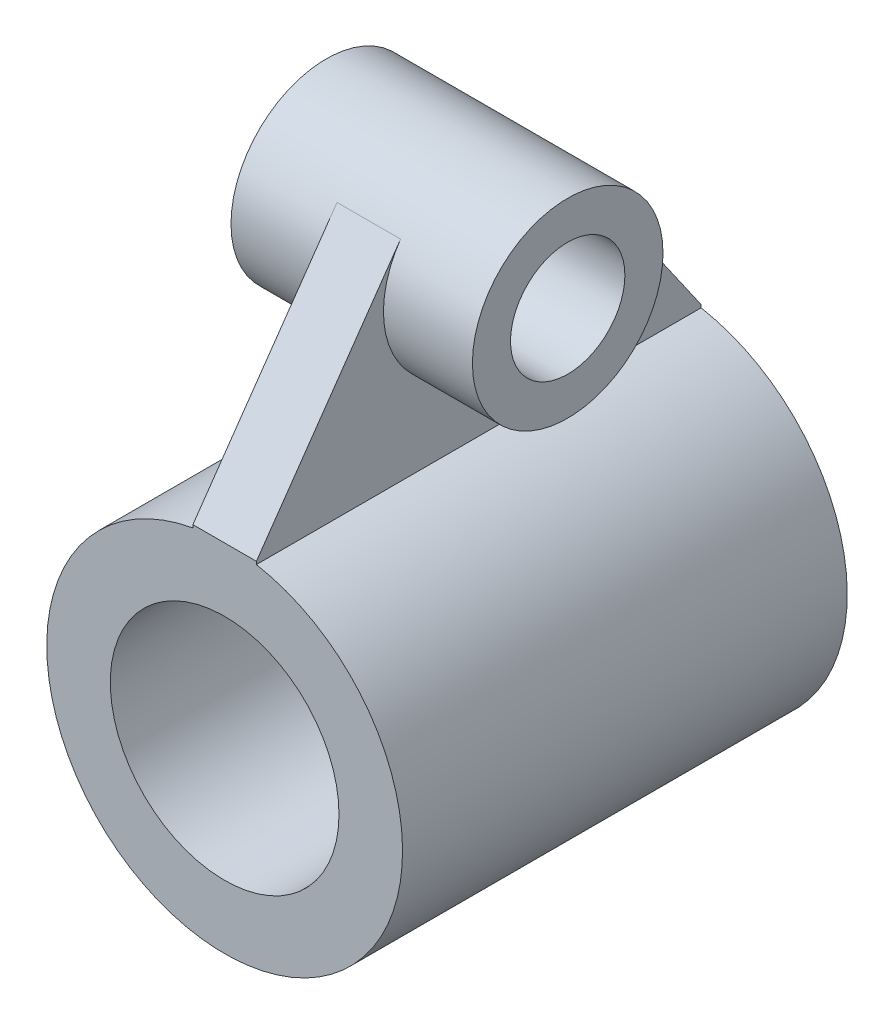
ISO-10303-21;
HEADER;
FILE_DESCRIPTION(('STEP AP214'),'2;1');
FILE_NAME('part.step','',(''),(''),'','','');
FILE_SCHEMA(('AUTOMOTIVE_DESIGN { 1 0 10303 214 1 1 1 1 }'));
ENDSEC;
DATA;
#1=APPLICATION_CONTEXT('core data for automotive mechanical design processes');
#2=APPLICATION_PROTOCOL_DEFINITION('international standard','automotive_design',2000,#1);
#3=PRODUCT_CONTEXT('',#1,'mechanical');
#4=PRODUCT('Part','Part','',(#3));
#5=PRODUCT_RELATED_PRODUCT_CATEGORY('part','',(#4));
#6=PRODUCT_DEFINITION_FORMATION('','',#4);
#7=PRODUCT_DEFINITION_CONTEXT('part definition',#1,'design');
#8=PRODUCT_DEFINITION('design','',#6,#7);
#9=PRODUCT_DEFINITION_SHAPE('','',#8);
#10=(LENGTH_UNIT() NAMED_UNIT(*) SI_UNIT(.MILLI.,.METRE.));
#11=(NAMED_UNIT(*) PLANE_ANGLE_UNIT() SI_UNIT($,.RADIAN.));
#12=(NAMED_UNIT(*) SI_UNIT($,.STERADIAN.) SOLID_ANGLE_UNIT());
#13=UNCERTAINTY_MEASURE_WITH_UNIT(LENGTH_MEASURE(1.E-05),#10,'distance_accuracy_value','');
#14=(GEOMETRIC_REPRESENTATION_CONTEXT(3) GLOBAL_UNCERTAINTY_ASSIGNED_CONTEXT((#13)) GLOBAL_UNIT_ASSIGNED_CONTEXT((#10,
#11,#12)) REPRESENTATION_CONTEXT('',''));
#15=CARTESIAN_POINT('',(0.,0.,0.));
#16=DIRECTION('',(0.,0.,1.));
#17=DIRECTION('',(1.,0.,0.));
#18=AXIS2_PLACEMENT_3D('',#15,#16,#17);
#19=CARTESIAN_POINT('',(0.,0.,-17.5));
#20=DIRECTION('',(0.,0.,1.));
#21=DIRECTION('',(1.,0.,0.));
#22=AXIS2_PLACEMENT_3D('',#19,#20,#21);
#23=CYLINDRICAL_SURFACE('',#22,14.);
#24=DIRECTION('',(0.,0.,1.));
#25=VECTOR('',#24,1.);
#26=CARTESIAN_POINT('',(2.5,13.7749773139559,-17.5));
#27=LINE('',#26,#25);
#28=CARTESIAN_POINT('',(2.5,13.7749773139559,17.5));
#29=VERTEX_POINT('',#28);
#30=CARTESIAN_POINT('',(2.5,13.7749773139559,-17.5));
#31=VERTEX_POINT('',#30);
#32=EDGE_CURVE('E61',#29,#31,#27,.F.);
#33=ORIENTED_EDGE('',*,*,#32,.F.);
#34=CARTESIAN_POINT('',(0.,0.,17.5));
#35=DIRECTION('',(0.,0.,1.));
#36=DIRECTION('',(1.,0.,0.));
#37=AXIS2_PLACEMENT_3D('',#34,#35,#36);
#38=CIRCLE('',#37,14.);
#39=CARTESIAN_POINT('',(-2.5,13.7749773139559,17.5));
#40=VERTEX_POINT('',#39);
#41=EDGE_CURVE('E48',#40,#29,#38,.T.);
#42=ORIENTED_EDGE('',*,*,#41,.F.);
#43=DIRECTION('',(0.,0.,1.));
#44=VECTOR('',#43,1.);
#45=CARTESIAN_POINT('',(-2.5,13.7749773139559,-17.5));
#46=LINE('',#45,#44);
#47=CARTESIAN_POINT('',(-2.5,13.7749773139559,-17.5));
#48=VERTEX_POINT('',#47);
#49=EDGE_CURVE('E115',#40,#48,#46,.F.);
#50=ORIENTED_EDGE('',*,*,#49,.T.);
#51=CARTESIAN_POINT('',(0.,0.,-17.5));
#52=DIRECTION('',(0.,0.,1.));
#53=DIRECTION('',(1.,0.,0.));
#54=AXIS2_PLACEMENT_3D('',#51,#52,#53);
#55=CIRCLE('',#54,14.);
#56=EDGE_CURVE('E11',#48,#31,#55,.T.);
#57=ORIENTED_EDGE('',*,*,#56,.T.);
#58=EDGE_LOOP('',(#33,#42,#50,#57));
#59=FACE_BOUND('',#58,.T.);
#60=ADVANCED_FACE('F41',(#59),#23,.T.);
#61=CARTESIAN_POINT('',(0.,0.,-17.5));
#62=DIRECTION('',(0.,0.,1.));
#63=DIRECTION('',(1.,0.,0.));
#64=AXIS2_PLACEMENT_3D('',#61,#62,#63);
#65=PLANE('',#64);
#66=ORIENTED_EDGE('',*,*,#56,.F.);
#67=DIRECTION('',(0.,1.,0.));
#68=VECTOR('',#67,1.);
#69=CARTESIAN_POINT('',(-2.5,0.,-17.5));
#70=LINE('',#69,#68);
#71=CARTESIAN_POINT('',(-2.5,14.,-17.5));
#72=VERTEX_POINT('',#71);
#73=EDGE_CURVE('E54',#48,#72,#70,.T.);
#74=ORIENTED_EDGE('',*,*,#73,.T.);
#75=DIRECTION('',(-1.,0.,0.));
#76=VECTOR('',#75,1.);
#77=CARTESIAN_POINT('',(2.5,14.,-17.5));
#78=LINE('',#77,#76);
#79=CARTESIAN_POINT('',(2.5,14.,-17.5));
#80=VERTEX_POINT('',#79);
#81=EDGE_CURVE('E126',#80,#72,#78,.T.);
#82=ORIENTED_EDGE('',*,*,#81,.F.);
#83=DIRECTION('',(0.,1.,0.));
#84=VECTOR('',#83,1.);
#85=CARTESIAN_POINT('',(2.5,0.,-17.5));
#86=LINE('',#85,#84);
#87=EDGE_CURVE('E155',#31,#80,#86,.T.);
#88=ORIENTED_EDGE('',*,*,#87,.F.);
#89=EDGE_LOOP('',(#66,#74,#82,#88));
#90=FACE_BOUND('',#89,.T.);
#91=CARTESIAN_POINT('',(0.,0.,-17.5));
#92=DIRECTION('',(0.,0.,1.));
#93=DIRECTION('',(1.,0.,0.));
#94=AXIS2_PLACEMENT_3D('',#91,#92,#93);
#95=CIRCLE('',#94,9.);
#96=CARTESIAN_POINT('',(9.,0.,-17.5));
#97=VERTEX_POINT('',#96);
#98=EDGE_CURVE('E134',#97,#97,#95,.T.);
#99=ORIENTED_EDGE('',*,*,#98,.T.);
#100=EDGE_LOOP('',(#99));
#101=FACE_BOUND('',#100,.T.);
#102=ADVANCED_FACE('F149',(#90,#101),#65,.F.);
#103=CARTESIAN_POINT('',(0.,0.,17.5));
#104=DIRECTION('',(0.,0.,1.));
#105=DIRECTION('',(1.,0.,0.));
#106=AXIS2_PLACEMENT_3D('',#103,#104,#105);
#107=PLANE('',#106);
#108=ORIENTED_EDGE('',*,*,#41,.T.);
#109=DIRECTION('',(0.,-1.,0.));
#110=VECTOR('',#109,1.);
#111=CARTESIAN_POINT('',(2.5,0.,17.5));
#112=LINE('',#111,#110);
#113=CARTESIAN_POINT('',(2.5,14.,17.5));
#114=VERTEX_POINT('',#113);
#115=EDGE_CURVE('E144',#114,#29,#112,.T.);
#116=ORIENTED_EDGE('',*,*,#115,.F.);
#117=DIRECTION('',(-1.,0.,0.));
#118=VECTOR('',#117,1.);
#119=CARTESIAN_POINT('',(2.5,14.,17.5));
#120=LINE('',#119,#118);
#121=CARTESIAN_POINT('',(-2.5,14.,17.5));
#122=VERTEX_POINT('',#121);
#123=EDGE_CURVE('E114',#114,#122,#120,.T.);
#124=ORIENTED_EDGE('',*,*,#123,.T.);
#125=DIRECTION('',(0.,-1.,0.));
#126=VECTOR('',#125,1.);
#127=CARTESIAN_POINT('',(-2.5,0.,17.5));
#128=LINE('',#127,#126);
#129=EDGE_CURVE('E116',#122,#40,#128,.T.);
#130=ORIENTED_EDGE('',*,*,#129,.T.);
#131=EDGE_LOOP('',(#108,#116,#124,#130));
#132=FACE_BOUND('',#131,.T.);
#133=CARTESIAN_POINT('',(0.,0.,17.5));
#134=DIRECTION('',(0.,0.,1.));
#135=DIRECTION('',(1.,0.,0.));
#136=AXIS2_PLACEMENT_3D('',#133,#134,#135);
#137=CIRCLE('',#136,9.);
#138=CARTESIAN_POINT('',(9.,0.,17.5));
#139=VERTEX_POINT('',#138);
#140=EDGE_CURVE('E132',#139,#139,#137,.T.);
#141=ORIENTED_EDGE('',*,*,#140,.F.);
#142=EDGE_LOOP('',(#141));
#143=FACE_BOUND('',#142,.T.);
#144=ADVANCED_FACE('F141',(#132,#143),#107,.T.);
#145=CARTESIAN_POINT('',(0.,0.,-17.5));
#146=DIRECTION('',(0.,0.,1.));
#147=DIRECTION('',(1.,0.,0.));
#148=AXIS2_PLACEMENT_3D('',#145,#146,#147);
#149=CYLINDRICAL_SURFACE('',#148,9.);
#150=ORIENTED_EDGE('',*,*,#98,.F.);
#151=EDGE_LOOP('',(#150));
#152=FACE_BOUND('',#151,.T.);
#153=ORIENTED_EDGE('',*,*,#140,.T.);
#154=EDGE_LOOP('',(#153));
#155=FACE_BOUND('',#154,.T.);
#156=ADVANCED_FACE('F203',(#152,#155),#149,.F.);
#157=CARTESIAN_POINT('',(2.5,12.7820709286032,18.3484454875048));
#158=DIRECTION('',(0.,0.57160484557998,0.820529036969129));
#159=DIRECTION('',(0.,-0.820529036969129,0.57160484557998));
#160=AXIS2_PLACEMENT_3D('',#157,#158,#159);
#161=PLANE('',#160);
#162=DIRECTION('',(0.,0.820529036969129,-0.57160484557998));
#163=VECTOR('',#162,1.);
#164=CARTESIAN_POINT('',(-2.5,12.7820709286032,18.3484454875048));
#165=LINE('',#164,#163);
#166=CARTESIAN_POINT('',(-2.5,30.2870363418499,6.15396777726847));
#167=VERTEX_POINT('',#166);
#168=EDGE_CURVE('E103',#122,#167,#165,.T.);
#169=ORIENTED_EDGE('',*,*,#168,.F.);
#170=ORIENTED_EDGE('',*,*,#123,.F.);
#171=DIRECTION('',(0.,0.820529036969129,-0.57160484557998));
#172=VECTOR('',#171,1.);
#173=CARTESIAN_POINT('',(2.5,12.7820709286032,18.3484454875048));
#174=LINE('',#173,#172);
#175=CARTESIAN_POINT('',(2.5,30.2870363418499,6.15396777726847));
#176=VERTEX_POINT('',#175);
#177=EDGE_CURVE('E112',#114,#176,#174,.T.);
#178=ORIENTED_EDGE('',*,*,#177,.T.);
#179=DIRECTION('',(-1.,0.,0.));
#180=VECTOR('',#179,1.);
#181=CARTESIAN_POINT('',(2.5,30.2870363418499,6.15396777726847));
#182=LINE('',#181,#180);
#183=EDGE_CURVE('E100',#176,#167,#182,.T.);
#184=ORIENTED_EDGE('',*,*,#183,.T.);
#185=EDGE_LOOP('',(#169,#170,#178,#184));
#186=FACE_BOUND('',#185,.T.);
#187=ADVANCED_FACE('F108',(#186),#161,.T.);
#188=CARTESIAN_POINT('',(2.5,12.7820709286032,-18.3484454875048));
#189=DIRECTION('',(0.,-0.57160484557998,0.820529036969129));
#190=DIRECTION('',(0.,-0.820529036969129,-0.57160484557998));
#191=AXIS2_PLACEMENT_3D('',#188,#189,#190);
#192=PLANE('',#191);
#193=DIRECTION('',(0.,0.820529036969129,0.57160484557998));
#194=VECTOR('',#193,1.);
#195=CARTESIAN_POINT('',(-2.5,12.7820709286032,-18.3484454875048));
#196=LINE('',#195,#194);
#197=CARTESIAN_POINT('',(-2.5,30.2870363418499,-6.15396777726847));
#198=VERTEX_POINT('',#197);
#199=EDGE_CURVE('E123',#72,#198,#196,.T.);
#200=ORIENTED_EDGE('',*,*,#199,.T.);
#201=DIRECTION('',(-1.,0.,0.));
#202=VECTOR('',#201,1.);
#203=CARTESIAN_POINT('',(2.5,30.2870363418499,-6.15396777726847));
#204=LINE('',#203,#202);
#205=CARTESIAN_POINT('',(2.5,30.2870363418499,-6.15396777726847));
#206=VERTEX_POINT('',#205);
#207=EDGE_CURVE('E99',#206,#198,#204,.T.);
#208=ORIENTED_EDGE('',*,*,#207,.F.);
#209=DIRECTION('',(0.,0.820529036969129,0.57160484557998));
#210=VECTOR('',#209,1.);
#211=CARTESIAN_POINT('',(2.5,12.7820709286032,-18.3484454875048));
#212=LINE('',#211,#210);
#213=EDGE_CURVE('E129',#80,#206,#212,.T.);
#214=ORIENTED_EDGE('',*,*,#213,.F.);
#215=ORIENTED_EDGE('',*,*,#81,.T.);
#216=EDGE_LOOP('',(#200,#208,#214,#215));
#217=FACE_BOUND('',#216,.T.);
#218=ADVANCED_FACE('F208',(#217),#192,.F.);
#219=CARTESIAN_POINT('',(2.5,0.,0.));
#220=DIRECTION('',(1.,0.,0.));
#221=DIRECTION('',(0.,0.,-1.));
#222=AXIS2_PLACEMENT_3D('',#219,#220,#221);
#223=PLANE('',#222);
#224=ORIENTED_EDGE('',*,*,#115,.T.);
#225=ORIENTED_EDGE('',*,*,#32,.T.);
#226=ORIENTED_EDGE('',*,*,#87,.T.);
#227=ORIENTED_EDGE('',*,*,#213,.T.);
#228=CARTESIAN_POINT('',(2.5,26.,0.));
#229=DIRECTION('',(1.,0.,0.));
#230=DIRECTION('',(0.,0.,-1.));
#231=AXIS2_PLACEMENT_3D('',#228,#229,#230);
#232=CIRCLE('',#231,7.5);
#233=EDGE_CURVE('E127',#176,#206,#232,.T.);
#234=ORIENTED_EDGE('',*,*,#233,.F.);
#235=ORIENTED_EDGE('',*,*,#177,.F.);
#236=EDGE_LOOP('',(#224,#225,#226,#227,#234,#235));
#237=FACE_BOUND('',#236,.T.);
#238=ADVANCED_FACE('F211',(#237),#223,.T.);
#239=CARTESIAN_POINT('',(-2.5,0.,0.));
#240=DIRECTION('',(1.,0.,0.));
#241=DIRECTION('',(0.,0.,-1.));
#242=AXIS2_PLACEMENT_3D('',#239,#240,#241);
#243=PLANE('',#242);
#244=ORIENTED_EDGE('',*,*,#49,.F.);
#245=ORIENTED_EDGE('',*,*,#129,.F.);
#246=ORIENTED_EDGE('',*,*,#168,.T.);
#247=CARTESIAN_POINT('',(-2.5,26.,0.));
#248=DIRECTION('',(1.,0.,0.));
#249=DIRECTION('',(0.,0.,-1.));
#250=AXIS2_PLACEMENT_3D('',#247,#248,#249);
#251=CIRCLE('',#250,7.5);
#252=EDGE_CURVE('E91',#167,#198,#251,.T.);
#253=ORIENTED_EDGE('',*,*,#252,.T.);
#254=ORIENTED_EDGE('',*,*,#199,.F.);
#255=ORIENTED_EDGE('',*,*,#73,.F.);
#256=EDGE_LOOP('',(#244,#245,#246,#253,#254,#255));
#257=FACE_BOUND('',#256,.T.);
#258=ADVANCED_FACE('F118',(#257),#243,.F.);
#259=CARTESIAN_POINT('',(9.5,26.,0.));
#260=DIRECTION('',(-1.,0.,0.));
#261=DIRECTION('',(0.,0.,1.));
#262=AXIS2_PLACEMENT_3D('',#259,#260,#261);
#263=CYLINDRICAL_SURFACE('',#262,7.5);
#264=ORIENTED_EDGE('',*,*,#233,.T.);
#265=ORIENTED_EDGE('',*,*,#207,.T.);
#266=ORIENTED_EDGE('',*,*,#252,.F.);
#267=ORIENTED_EDGE('',*,*,#183,.F.);
#268=EDGE_LOOP('',(#264,#265,#266,#267));
#269=FACE_BOUND('',#268,.T.);
#270=CARTESIAN_POINT('',(9.5,26.,0.));
#271=DIRECTION('',(1.,0.,0.));
#272=DIRECTION('',(0.,0.,-1.));
#273=AXIS2_PLACEMENT_3D('',#270,#271,#272);
#274=CIRCLE('',#273,7.5);
#275=CARTESIAN_POINT('',(9.5,26.,-7.5));
#276=VERTEX_POINT('',#275);
#277=EDGE_CURVE('E102',#276,#276,#274,.T.);
#278=ORIENTED_EDGE('',*,*,#277,.F.);
#279=EDGE_LOOP('',(#278));
#280=FACE_BOUND('',#279,.T.);
#281=CARTESIAN_POINT('',(-9.5,26.,0.));
#282=DIRECTION('',(1.,0.,0.));
#283=DIRECTION('',(0.,0.,-1.));
#284=AXIS2_PLACEMENT_3D('',#281,#282,#283);
#285=CIRCLE('',#284,7.5);
#286=CARTESIAN_POINT('',(-9.5,26.,-7.5));
#287=VERTEX_POINT('',#286);
#288=EDGE_CURVE('E162',#287,#287,#285,.T.);
#289=ORIENTED_EDGE('',*,*,#288,.T.);
#290=EDGE_LOOP('',(#289));
#291=FACE_BOUND('',#290,.T.);
#292=ADVANCED_FACE('F92',(#269,#280,#291),#263,.T.);
#293=CARTESIAN_POINT('',(9.5,26.,0.));
#294=DIRECTION('',(1.,0.,0.));
#295=DIRECTION('',(0.,0.,-1.));
#296=AXIS2_PLACEMENT_3D('',#293,#294,#295);
#297=PLANE('',#296);
#298=CARTESIAN_POINT('',(9.5,26.,0.));
#299=DIRECTION('',(1.,0.,0.));
#300=DIRECTION('',(0.,0.,-1.));
#301=AXIS2_PLACEMENT_3D('',#298,#299,#300);
#302=CIRCLE('',#301,4.5);
#303=CARTESIAN_POINT('',(9.5,26.,-4.5));
#304=VERTEX_POINT('',#303);
#305=EDGE_CURVE('E163',#304,#304,#302,.T.);
#306=ORIENTED_EDGE('',*,*,#305,.F.);
#307=EDGE_LOOP('',(#306));
#308=FACE_BOUND('',#307,.T.);
#309=ORIENTED_EDGE('',*,*,#277,.T.);
#310=EDGE_LOOP('',(#309));
#311=FACE_BOUND('',#310,.T.);
#312=ADVANCED_FACE('F174',(#308,#311),#297,.T.);
#313=CARTESIAN_POINT('',(-9.5,26.,0.));
#314=DIRECTION('',(1.,0.,0.));
#315=DIRECTION('',(0.,0.,-1.));
#316=AXIS2_PLACEMENT_3D('',#313,#314,#315);
#317=PLANE('',#316);
#318=CARTESIAN_POINT('',(-9.5,26.,0.));
#319=DIRECTION('',(1.,0.,0.));
#320=DIRECTION('',(0.,0.,-1.));
#321=AXIS2_PLACEMENT_3D('',#318,#319,#320);
#322=CIRCLE('',#321,4.5);
#323=CARTESIAN_POINT('',(-9.5,26.,-4.5));
#324=VERTEX_POINT('',#323);
#325=EDGE_CURVE('E159',#324,#324,#322,.T.);
#326=ORIENTED_EDGE('',*,*,#325,.T.);
#327=EDGE_LOOP('',(#326));
#328=FACE_BOUND('',#327,.T.);
#329=ORIENTED_EDGE('',*,*,#288,.F.);
#330=EDGE_LOOP('',(#329));
#331=FACE_BOUND('',#330,.T.);
#332=ADVANCED_FACE('F180',(#328,#331),#317,.F.);
#333=CARTESIAN_POINT('',(-14.,26.,0.));
#334=DIRECTION('',(1.,0.,0.));
#335=DIRECTION('',(0.,0.,-1.));
#336=AXIS2_PLACEMENT_3D('',#333,#334,#335);
#337=CYLINDRICAL_SURFACE('',#336,4.5);
#338=ORIENTED_EDGE('',*,*,#305,.T.);
#339=EDGE_LOOP('',(#338));
#340=FACE_BOUND('',#339,.T.);
#341=ORIENTED_EDGE('',*,*,#325,.F.);
#342=EDGE_LOOP('',(#341));
#343=FACE_BOUND('',#342,.T.);
#344=ADVANCED_FACE('F175',(#340,#343),#337,.F.);
#345=CLOSED_SHELL('',(#60,#102,#144,#156,#187,#218,#238,#258,#292,#312,#332,#344));
#346=MANIFOLD_SOLID_BREP('B2',#345);
#347=ADVANCED_BREP_SHAPE_REPRESENTATION('',(#18,#346),#14);
#348=SHAPE_DEFINITION_REPRESENTATION(#9,#347);
ENDSEC;
END-ISO-10303-21;
